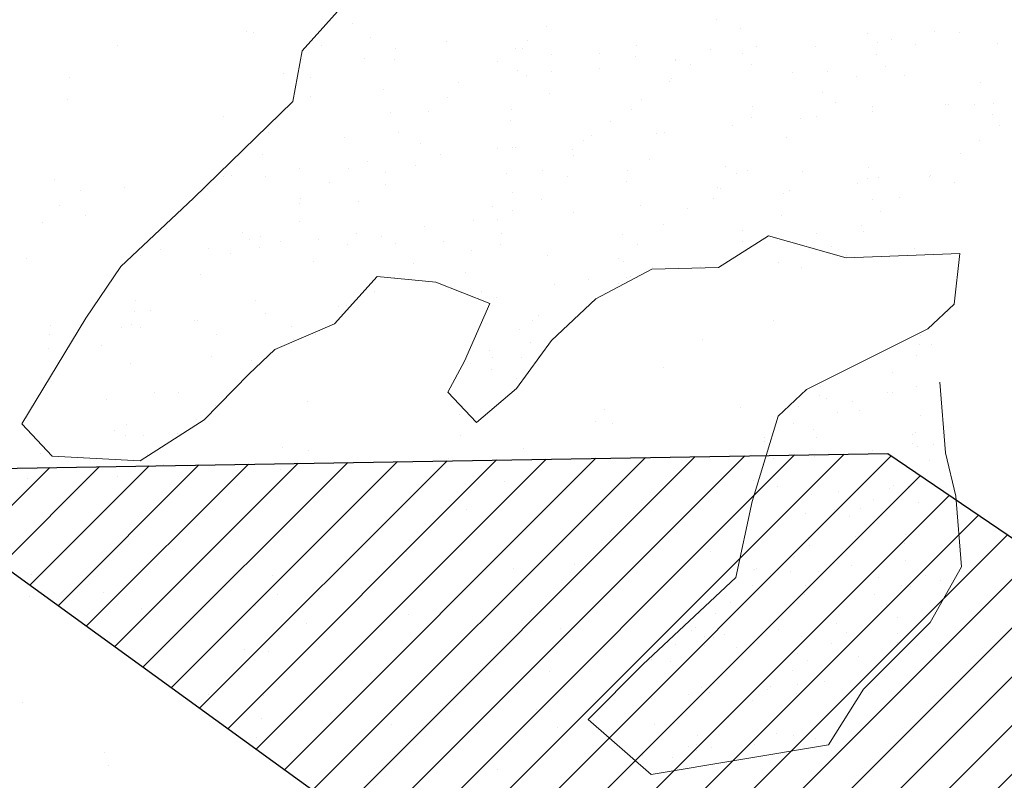
# Model space of a CAD drawing. Units: inches. Extents: x 1986 to 21484, y -1816 to 2016.
# Tile 61 of 85: x 3651.423 to 3655.81, y 1889.501 to 1892.891. Entities that reach past the tile are written whole.
import ezdxf

# ---------------------------------------------------------------- set-up
doc = ezdxf.new("R2010")
doc.units = ezdxf.units.IN
doc.layers.add('L-PLNT', color=84, linetype='Continuous', lineweight=13)
doc.layers.add('vfolha2', color=110, linetype='Continuous')

# ---------------------------------------------------------------- blocks, each defined once
blk = doc.blocks.new('arbusto_PB_verde_grande')
at = {"layer": 'vfolha2'}
h = blk.add_hatch(dxfattribs=at)
h.set_pattern_fill('ANSI31', color=256, scale=0.05, style=0)
h.set_pattern_definition([(45, (-2446.5133113, 50.986076), (-0.004419417382, 0.004419417382), [])])
h.paths.add_polyline_path([(0.02944, 0.35651), (0.00028, 0.09048), (0.02625, -0.03934), (0.047, 0.06233), (0.06189, 0.09731), (0.09372, 0.26573), (0.09955, 0.43473), (0.08789, 0.61313), (0.0645, 0.72266), (0.04988, 0.6851), (0.0236, 0.51294)])
h.paths.add_polyline_path([(0.30106, 0.43789), (0.14225, 0.24871), (0.26685, 0.30022)])
h.paths.add_polyline_path([(0.37995, 0.22817), (0.23697, 0.15193), (0.18428, 0.09364), (0.11122, 0.04358), (0.02625, -0.03934), (0.28061, 0.04667), (0.36829, 0.07798), (0.46756, 0.11239), (0.61068, 0.19376), (0.71585, 0.27823), (0.55813, 0.25948)])
h.paths.add_polyline_path([(0.56101, -0.29441), (0.72752, -0.32573), (0.59024, -0.2412), (0.42962, -0.15982), (0.02625, -0.03934), (0.14922, -0.14107), (0.18838, -0.16604), (0.41501, -0.24435)])
h.paths.add_polyline_path([(-0.27429, -0.44776), (-0.30352, -0.72628), (-0.23923, -0.64175), (-0.15457, -0.45716), (0.02625, -0.03934), (-0.16328, -0.25376)])
h.paths.add_polyline_path([(-0.51963, -0.24744), (-0.67736, -0.32573), (-0.59558, -0.35072), (-0.40574, -0.32882), (-0.21007, -0.20995), (0.02625, -0.03934), (-0.14874, -0.06595), (-0.31518, -0.09101), (-0.41452, -0.15048)])
h.paths.add_polyline_path([(-0.52546, 0.25007), (-0.70947, 0.24698), (-0.51963, 0.1093), (-0.32979, 0.02167), (-0.07567, -0.0128), (-0.04234, -0.02148), (-0.35024, 0.1312)])
for p, q in [((-0.70947, 0.24698), (-0.52546, 0.25007)), ((-0.52546, 0.25007), (-0.35024, 0.1312)), ((-0.51963, 0.1093), (-0.70947, 0.24698))]:
    blk.add_line(p, q, dxfattribs=at)
blk = doc.blocks.new('PLANT-SHRUB')
for p, q in [((2170.2504, 1876.25), (2169.9665, 1876.176)), ((2170.9168, 1875.8061), (2170.2504, 1876.25)), ((2169.9665, 1876.176), (2169.5469, 1876.1637)), ((2170.2731, 1876.1911), (2170.2731, 1876.1911)), ((2169.5469, 1876.1637), (2169.2754, 1876.0773)), ((2169.5469, 1876.1637), (2169.5469, 1876.1637)), ((2169.7163, 1876.1281), (2169.7163, 1876.1281)), ((2169.6868, 1876.1011), (2169.6868, 1876.1011)), ((2170.336, 1876.1153), (2170.336, 1876.1153)), ((2169.2754, 1876.0773), (2169.0779, 1875.8307)), ((2169.387, 1876.0573), (2169.387, 1876.0573)), ((2169.6384, 1876.0466), (2169.6384, 1876.0466)), ((2169.8848, 1876.0564), (2169.8848, 1876.0564)), ((2170.3827, 1876.0555), (2170.3827, 1876.0555)), ((2169.4198, 1875.9977), (2169.4198, 1875.9977)), ((2170.0702, 1876.031), (2170.0702, 1876.031)), ((2170.4887, 1876.0257), (2170.4887, 1876.0257)), ((2169.503, 1875.9867), (2169.503, 1875.9867)), ((2169.5277, 1875.9553), (2169.5277, 1875.9553)), ((2169.633, 1875.9696), (2169.633, 1875.9696)), ((2170.1674, 1875.9608), (2170.1674, 1875.9608)), ((2170.1969, 1875.9878), (2170.1969, 1875.9878)), ((2169.8501, 1875.941), (2169.8501, 1875.941)), ((2169.9334, 1875.9301), (2169.9334, 1875.9301)), ((2170.0633, 1875.913), (2170.0633, 1875.913)), ((2169.4356, 1875.8865), (2169.4356, 1875.8865)), ((2169.6421, 1875.9018), (2169.6421, 1875.9018)), ((2169.8541, 1875.8811), (2169.8541, 1875.8811)), ((2170.14, 1875.9009), (2170.14, 1875.9009)), ((2170.263, 1875.8831), (2170.263, 1875.8831)), ((2170.2805, 1875.8844), (2170.2805, 1875.8844)), ((2170.3637, 1875.8734), (2170.3637, 1875.8734)), ((2170.6378, 1875.9), (2170.6378, 1875.9)), ((2170.6948, 1875.8675), (2170.6948, 1875.8675)), ((2169.0779, 1875.8307), (2168.9792, 1875.6581)), ((2169.3886, 1875.8279), (2169.3886, 1875.8279)), ((2169.5747, 1875.8588), (2169.5747, 1875.8588)), ((2170.0725, 1875.8579), (2170.0725, 1875.8579)), ((2170.4937, 1875.8563), (2170.4937, 1875.8563)), ((2170.5704, 1875.857), (2170.5704, 1875.857)), ((2170.648, 1875.8205), (2170.648, 1875.8205)), ((2170.6775, 1875.8475), (2170.6775, 1875.8475)), ((2170.7108, 1875.8277), (2170.7108, 1875.8277)), ((2169.3592, 1875.8009), (2169.3592, 1875.8009)), ((2170.0083, 1875.815), (2170.0083, 1875.815)), ((2170.794, 1875.8168), (2170.794, 1875.8168)), ((2170.9538, 1875.4361), (2170.9168, 1875.8061)), ((2169.2194, 1875.7366), (2169.2194, 1875.7366)), ((2169.6284, 1875.7385), (2169.6284, 1875.7385)), ((2169.8692, 1875.6876), (2169.8692, 1875.6876)), ((2170.0602, 1875.723), (2170.0602, 1875.723)), ((2170.4786, 1875.7176), (2170.4786, 1875.7176)), ((2170.8876, 1875.7196), (2170.8876, 1875.7196)), ((2168.9792, 1875.6581), (2168.7818, 1875.4114)), ((2169.2001, 1875.6551), (2169.2001, 1875.6551)), ((2169.2578, 1875.657), (2169.2578, 1875.657)), ((2169.5298, 1875.6563), (2169.5298, 1875.6563)), ((2169.7557, 1875.6561), (2169.7557, 1875.6561)), ((2169.8398, 1875.6606), (2169.8398, 1875.6606)), ((2170.2535, 1875.6552), (2170.2535, 1875.6552)), ((2170.4889, 1875.6747), (2170.4889, 1875.6747)), ((2170.5522, 1875.6612), (2170.5522, 1875.6612)), ((2170.7514, 1875.6543), (2170.7514, 1875.6543)), ((2169.0553, 1875.6318), (2169.0553, 1875.6318)), ((2169.2502, 1875.6061), (2169.2502, 1875.6061)), ((2169.2724, 1875.6032), (2169.2724, 1875.6032)), ((2168.9937, 1875.594), (2168.9937, 1875.594)), ((2169.3556, 1875.5922), (2169.3556, 1875.5922)), ((2169.4255, 1875.5784), (2169.4255, 1875.5784)), ((2169.4856, 1875.5751), (2169.4856, 1875.5751)), ((2169.844, 1875.5731), (2169.844, 1875.5731)), ((2170.2529, 1875.575), (2170.2529, 1875.575)), ((2170.6847, 1875.5595), (2170.6847, 1875.5595)), ((2169.05, 1875.5534), (2169.05, 1875.5534)), ((2169.061, 1875.5276), (2169.061, 1875.5276)), ((2169.6806, 1875.5148), (2169.6806, 1875.5148)), ((2169.7027, 1875.5465), (2169.7027, 1875.5465)), ((2169.786, 1875.5356), (2169.786, 1875.5356)), ((2169.7931, 1875.5346), (2169.7931, 1875.5346)), ((2169.9159, 1875.5185), (2169.9159, 1875.5185)), ((2170.2946, 1875.5512), (2170.2946, 1875.5512)), ((2170.3203, 1875.5203), (2170.3203, 1875.5203)), ((2170.3498, 1875.5473), (2170.3498, 1875.5473)), ((2169.0151, 1875.5024), (2169.0151, 1875.5024)), ((2169.0315, 1875.5006), (2169.0315, 1875.5006)), ((2169.513, 1875.5015), (2169.513, 1875.5015)), ((2170.0108, 1875.5005), (2170.0108, 1875.5005)), ((2170.1331, 1875.4899), (2170.1331, 1875.4899)), ((2170.2163, 1875.4789), (2170.2163, 1875.4789)), ((2170.5087, 1875.4996), (2170.5087, 1875.4996)), ((2168.9477, 1875.4594), (2168.9477, 1875.4594)), ((2169.2093, 1875.4285), (2169.2093, 1875.4285)), ((2169.4456, 1875.4585), (2169.4456, 1875.4585)), ((2169.6183, 1875.4305), (2169.6183, 1875.4305)), ((2169.7567, 1875.2265), (2170.0406, 1875.4238)), ((2169.9434, 1875.4576), (2169.9434, 1875.4576)), ((2169.9553, 1875.456), (2169.9553, 1875.456)), ((2170.0406, 1875.4238), (2170.6083, 1875.4238)), ((2170.326, 1875.4645), (2170.326, 1875.4645)), ((2170.3463, 1875.4618), (2170.3463, 1875.4618)), ((2170.4413, 1875.4567), (2170.4413, 1875.4567)), ((2170.5634, 1875.4332), (2170.5634, 1875.4332)), ((2170.6083, 1875.4238), (2170.9538, 1875.4361)), ((2170.9391, 1875.4558), (2170.9391, 1875.4558)), ((2169.5416, 1875.3873), (2169.5416, 1875.3873)), ((2170.8689, 1875.393), (2170.8689, 1875.393)), ((2168.8724, 1875.3548), (2168.8724, 1875.3548)), ((2169.5121, 1875.3603), (2169.5121, 1875.3603)), ((2171.0769, 1875.3656), (2171.0769, 1875.3656)), ((2168.9656, 1875.2998), (2168.9656, 1875.2998)), ((2171.4019, 1875.3228), (2171.4019, 1875.3228)), ((2168.6947, 1875.2653), (2168.6947, 1875.2653)), ((2168.7779, 1875.2544), (2168.7779, 1875.2544)), ((2168.9837, 1875.2859), (2168.9837, 1875.2859)), ((2169.1287, 1875.2566), (2169.1287, 1875.2566)), ((2169.4154, 1875.2704), (2169.4154, 1875.2704)), ((2169.6266, 1875.2557), (2169.6266, 1875.2557)), ((2170.0451, 1875.2609), (2170.0451, 1875.2609)), ((2171.0912, 1875.2476), (2171.0912, 1875.2476)), ((2168.7333, 1875.2274), (2168.7333, 1875.2274)), ((2168.9079, 1875.2372), (2168.9079, 1875.2372)), ((2169.125, 1875.2087), (2169.125, 1875.2087)), ((2169.353, 1875.2145), (2169.353, 1875.2145)), ((2169.4112, 1875.0292), (2169.7567, 1875.2265)), ((2168.3251, 1875.0538), (2168.4979, 1875.2018)), ((2168.4979, 1875.2018), (2168.6583, 1875.2018)), ((2168.6583, 1875.2018), (2169.2384, 1875.0292)), ((2168.7038, 1875.2004), (2168.7038, 1875.2004)), ((2169.2082, 1875.1977), (2169.2082, 1875.1977)), ((2169.3382, 1875.1806), (2169.3382, 1875.1806)), ((2169.6879, 1875.1646), (2169.6879, 1875.1646)), ((2170.9325, 1875.1624), (2170.9325, 1875.1624)), ((2169.1993, 1875.1205), (2169.1993, 1875.1205)), ((2169.5553, 1875.152), (2169.5553, 1875.152)), ((2169.6075, 1875.1374), (2169.6075, 1875.1374)), ((2169.2139, 1875.0871), (2169.2139, 1875.0871)), ((2169.3839, 1875.1011), (2169.3839, 1875.1011)), ((2171.1567, 1875.1052), (2171.1567, 1875.1052)), ((2168.3251, 1875.0538), (2168.3251, 1875.0538)), ((2168.7077, 1874.7209), (2168.3251, 1875.0538)), ((2169.1844, 1875.0601), (2169.1844, 1875.0601)), ((2169.2384, 1875.0292), (2169.4112, 1875.0292)), ((2169.3165, 1875.0582), (2169.3165, 1875.0582)), ((2169.5194, 1875.0573), (2169.5194, 1875.0573)), ((2169.5339, 1875.0699), (2169.5339, 1875.0699)), ((2170.764, 1875.055), (2170.764, 1875.055)), ((2168.4584, 1874.8995), (2168.4584, 1874.8995)), ((2168.4584, 1874.8995), (2168.4584, 1874.8995)), ((2169.5046, 1874.8862), (2169.5046, 1874.8862)), ((2170.527, 1874.8911), (2170.527, 1874.8911)), ((2171.6065, 1874.8522), (2171.6065, 1874.8522)), ((2168.1245, 1874.8072), (2168.1245, 1874.8072)), ((2170.809, 1874.7866), (2170.809, 1874.7866)), ((2167.8059, 1874.7614), (2167.8059, 1874.7614)), ((2167.9149, 1874.7471), (2167.9149, 1874.7471)), ((2168.0189, 1874.7334), (2168.0189, 1874.7334)), ((2168.8928, 1874.4126), (2168.7077, 1874.7209)), ((2167.7959, 1874.7038), (2167.7959, 1874.7038)), ((2168.1814, 1874.712), (2168.1814, 1874.712)), ((2168.1882, 1874.7122), (2168.1882, 1874.7122)), ((2168.3488, 1874.69), (2168.3488, 1874.69)), ((2168.5705, 1874.6877), (2168.5705, 1874.6877)), ((2168.6994, 1874.7146), (2168.6994, 1874.7146)), ((2169.1361, 1874.7054), (2169.1361, 1874.7054)), ((2170.7353, 1874.7191), (2170.7353, 1874.7191)), ((2167.759, 1874.67), (2167.759, 1874.67)), ((2168.4528, 1874.6763), (2168.4528, 1874.6763)), ((2168.5568, 1874.6626), (2168.5568, 1874.6626)), ((2168.5568, 1874.6626), (2168.5568, 1874.6626)), ((2168.7193, 1874.6412), (2168.7193, 1874.6412)), ((2167.8211, 1874.6139), (2167.8211, 1874.6139)), ((2168.4434, 1874.6128), (2168.4434, 1874.6128)), ((2168.8817, 1874.6198), (2168.8817, 1874.6198)), ((2167.7368, 1874.5603), (2167.7368, 1874.5603)), ((2168.3591, 1874.5591), (2168.3591, 1874.5591)), ((2168.7272, 1874.5526), (2168.7272, 1874.5526)), ((2169.4246, 1874.5483), (2169.4246, 1874.5483)), ((2169.9719, 1874.5504), (2169.9719, 1874.5504)), ((2171.2165, 1874.5481), (2171.2165, 1874.5481)), ((2167.9061, 1874.5339), (2167.9061, 1874.5339)), ((2167.918, 1874.5248), (2167.918, 1874.5248)), ((2168.3966, 1874.5284), (2168.3966, 1874.5284)), ((2168.4459, 1874.5145), (2168.4459, 1874.5145)), ((2168.9404, 1874.5297), (2168.9404, 1874.5297)), ((2169.6326, 1874.5209), (2169.6326, 1874.5209)), ((2167.5601, 1874.4878), (2167.5601, 1874.4878)), ((2168.3598, 1874.4946), (2168.3598, 1874.4946)), ((2169.9576, 1874.4782), (2169.9576, 1874.4782)), ((2170.0199, 1874.4908), (2170.0199, 1874.4908)), ((2171.0661, 1874.4775), (2171.0661, 1874.4775)), ((2172.0884, 1874.4824), (2172.0884, 1874.4824)), ((2172.0105, 1874.4358), (2172.0105, 1874.4358)), ((2168.7884, 1874.3867), (2168.7884, 1874.3867)), ((2169.152, 1874.3632), (2168.8928, 1874.4126)), ((2170.5004, 1874.4067), (2170.5004, 1874.4067)), ((2170.7085, 1874.3793), (2170.7085, 1874.3793)), ((2167.6526, 1874.3338), (2167.6526, 1874.3338)), ((2168.1756, 1874.3271), (2168.1756, 1874.3271)), ((2168.6868, 1874.3296), (2168.6868, 1874.3296)), ((2168.9973, 1874.353), (2168.9973, 1874.353)), ((2169.3741, 1874.1659), (2169.152, 1874.3632)), ((2170.3375, 1874.3546), (2170.3375, 1874.3546)), ((2171.0334, 1874.3365), (2171.0334, 1874.3365)), ((2171.9368, 1874.3683), (2171.9368, 1874.3683)), ((2167.9631, 1874.3068), (2167.9631, 1874.3068)), ((2168.1609, 1874.3124), (2168.1609, 1874.3124)), ((2168.5854, 1874.3057), (2168.5854, 1874.3057)), ((2168.7147, 1874.3192), (2168.7147, 1874.3192)), ((2168.9605, 1874.3192), (2168.9605, 1874.3192)), ((2169.2077, 1874.3045), (2169.2077, 1874.3045)), ((2167.7306, 1874.2539), (2167.7306, 1874.2539)), ((2167.8346, 1874.2402), (2167.8346, 1874.2402)), ((2171.5762, 1874.2651), (2171.5762, 1874.2651)), ((2167.9971, 1874.2189), (2167.9971, 1874.2189)), ((2171.7843, 1874.2377), (2171.7843, 1874.2377)), ((2172.1092, 1874.1949), (2172.1092, 1874.1949)), ((2167.987, 1874.1531), (2167.987, 1874.1531)), ((2168.1205, 1874.1661), (2168.1205, 1874.1661)), ((2168.2685, 1874.1831), (2168.2685, 1874.1831)), ((2168.3726, 1874.1694), (2168.3726, 1874.1694)), ((2169.3651, 1874.1638), (2169.3651, 1874.1638)), ((2169.6456, 1874.0919), (2169.3741, 1874.1659)), ((2170.6097, 1874.1616), (2170.6097, 1874.1616)), ((2171.8544, 1874.1593), (2171.8544, 1874.1593)), ((2167.8935, 1874.1489), (2167.8935, 1874.1489)), ((2167.9502, 1874.1193), (2167.9502, 1874.1193)), ((2168.282, 1874.1124), (2168.282, 1874.1124)), ((2168.4333, 1874.1294), (2168.4333, 1874.1294)), ((2168.4333, 1874.1294), (2168.4333, 1874.1294)), ((2168.535, 1874.148), (2168.535, 1874.148)), ((2168.7616, 1874.137), (2168.7616, 1874.137)), ((2168.8065, 1874.1123), (2168.8065, 1874.1123)), ((2168.9043, 1874.1113), (2168.9043, 1874.1113)), ((2168.9564, 1874.1228), (2168.9564, 1874.1228)), ((2169.4676, 1874.1252), (2169.4676, 1874.1252)), ((2169.4794, 1874.1161), (2169.4794, 1874.1161)), ((2169.5266, 1874.1101), (2169.5266, 1874.1101)), ((2170.1763, 1874.1413), (2169.9172, 1874.0919)), ((2170.149, 1874.109), (2170.149, 1874.109)), ((2170.4108, 1874.1289), (2170.1763, 1874.1413)), ((2170.4108, 1874.1289), (2170.4108, 1874.1289)), ((2170.4108, 1873.944), (2170.4108, 1874.1289)), ((2170.5018, 1874.121), (2170.5018, 1874.121)), ((2172.6521, 1874.1234), (2172.6521, 1874.1234)), ((2168.9105, 1874.0986), (2168.9105, 1874.0986)), ((2169.0729, 1874.0772), (2169.0729, 1874.0772)), ((2169.9172, 1874.0919), (2169.6456, 1874.0919)), ((2170.0073, 1874.1058), (2170.0073, 1874.1058)), ((2171.5813, 1874.0821), (2171.5813, 1874.0821)), ((2172.6275, 1874.0688), (2172.6275, 1874.0688)), ((2167.9519, 1874.0587), (2167.9519, 1874.0587)), ((2168.1977, 1874.0587), (2168.1977, 1874.0587)), ((2168.8201, 1874.0576), (2168.8201, 1874.0576)), ((2169.1966, 1874.0565), (2169.1966, 1874.0565)), ((2169.3444, 1874.0415), (2169.3444, 1874.0415)), ((2169.4424, 1874.0565), (2169.4424, 1874.0565)), ((2169.4484, 1874.0278), (2169.4484, 1874.0278)), ((2169.9898, 1874.036), (2169.9898, 1874.036)), ((2170.0647, 1874.0553), (2170.0647, 1874.0553)), ((2170.4412, 1874.0542), (2170.4412, 1874.0542)), ((2171.6858, 1874.0519), (2171.6858, 1874.0519)), ((2168.5877, 1873.9777), (2168.5877, 1873.9777)), ((2169.6108, 1874.0064), (2169.6108, 1874.0064)), ((2170.1988, 1874.0022), (2170.1988, 1874.0022)), ((2171.539, 1874.0038), (2171.539, 1874.0038)), ((2168.1631, 1873.9421), (2168.1631, 1873.9421)), ((2168.3169, 1873.9547), (2168.3169, 1873.9547)), ((2168.5509, 1873.9439), (2168.5509, 1873.9439)), ((2168.6742, 1873.9445), (2168.6742, 1873.9445)), ((2169.3623, 1873.9616), (2169.3623, 1873.9616)), ((2169.8823, 1873.9707), (2169.8823, 1873.9707)), ((2169.9162, 1873.9685), (2169.9162, 1873.9685)), ((2169.9863, 1873.957), (2169.9863, 1873.957)), ((2170.1488, 1873.9356), (2170.1488, 1873.9356)), ((2170.162, 1873.9685), (2170.162, 1873.9685)), ((2170.2627, 1873.8946), (2170.4108, 1873.944)), ((2169.214, 1873.9251), (2169.214, 1873.9251)), ((2169.7371, 1873.9184), (2169.7371, 1873.9184)), ((2170.0035, 1873.7837), (2170.2627, 1873.8946)), ((2170.2483, 1873.9209), (2170.2483, 1873.9209)), ((2168.424, 1873.8053), (2168.424, 1873.8053)), ((2169.0463, 1873.8041), (2169.0463, 1873.8041)), ((2169.1885, 1873.8023), (2169.1885, 1873.8023)), ((2169.6686, 1873.803), (2169.6686, 1873.803)), ((2168.352, 1873.7617), (2168.352, 1873.7617)), ((2168.9152, 1873.7596), (2168.9152, 1873.7596)), ((2169.1516, 1873.7685), (2169.1516, 1873.7685)), ((2169.9631, 1873.7862), (2169.9631, 1873.7862)), ((2170.1146, 1873.5494), (2170.0035, 1873.7837)), ((2168.4207, 1873.7444), (2168.4207, 1873.7444)), ((2168.9438, 1873.7377), (2168.9438, 1873.7377)), ((2169.455, 1873.7402), (2169.455, 1873.7402)), ((2169.9947, 1873.7207), (2169.9947, 1873.7207)), ((2169.9947, 1873.7207), (2169.9947, 1873.7207)), ((2172.0633, 1873.7123), (2172.0633, 1873.7123)), ((2171.0409, 1873.7074), (2171.0409, 1873.7074)), ((2171.1913, 1873.6852), (2171.1913, 1873.6852)), ((2168.3508, 1873.6549), (2168.3508, 1873.6549)), ((2168.5132, 1873.6335), (2168.5132, 1873.6335)), ((2169.7892, 1873.6269), (2169.7892, 1873.6269)), ((2172.7405, 1873.653), (2172.7405, 1873.653)), ((2168.6222, 1873.6192), (2168.6222, 1873.6192)), ((2168.7262, 1873.6055), (2168.7262, 1873.6055)), ((2168.7429, 1873.6109), (2168.7429, 1873.6109)), ((2168.8887, 1873.5841), (2168.8887, 1873.5841)), ((2168.9527, 1873.5863), (2168.9527, 1873.5863)), ((2169.3653, 1873.6097), (2169.3653, 1873.6097)), ((2169.5184, 1873.6039), (2169.5184, 1873.6039)), ((2169.7524, 1873.5931), (2169.7524, 1873.5931)), ((2169.9876, 1873.6086), (2169.9876, 1873.6086)), ((2171.1176, 1873.6177), (2171.1176, 1873.6177)), ((2168.4044, 1873.5518), (2168.4044, 1873.5518)), ((2168.6587, 1873.5572), (2168.6587, 1873.5572)), ((2168.6617, 1873.5595), (2168.6617, 1873.5595)), ((2169.0561, 1873.562), (2169.0561, 1873.562)), ((2169.1601, 1873.5483), (2169.1601, 1873.5483)), ((2169.2014, 1873.54), (2169.2014, 1873.54)), ((2169.281, 1873.556), (2169.281, 1873.556)), ((2169.6491, 1873.5495), (2169.6491, 1873.5495)), ((2169.9033, 1873.5549), (2169.9033, 1873.5549)), ((2170.1146, 1873.5494), (2170.1146, 1873.5494)), ((2170.2874, 1873.352), (2170.1146, 1873.5494)), ((2170.8937, 1873.5473), (2170.8937, 1873.5473)), ((2172.1383, 1873.545), (2172.1383, 1873.545)), ((2169.2641, 1873.5346), (2169.2641, 1873.5346)), ((2169.2641, 1873.5346), (2169.2641, 1873.5346)), ((2169.4266, 1873.5133), (2169.4266, 1873.5133)), ((2169.7245, 1873.5334), (2169.7245, 1873.5334)), ((2169.5891, 1873.4919), (2169.5891, 1873.4919)), ((2169.698, 1873.4775), (2169.698, 1873.4775)), ((2169.802, 1873.4638), (2169.802, 1873.4638)), ((2168.7789, 1873.427), (2168.7789, 1873.427)), ((2169.5535, 1873.4109), (2169.5535, 1873.4109)), ((2169.9645, 1873.4424), (2169.9645, 1873.4424)), ((2170.1319, 1873.4204), (2170.1319, 1873.4204)), ((2170.2359, 1873.4067), (2170.2359, 1873.4067)), ((2168.742, 1873.3932), (2168.742, 1873.3932)), ((2170.5712, 1873.3767), (2170.2874, 1873.352)), ((2170.34, 1873.393), (2170.34, 1873.393)), ((2170.8427, 1873.2781), (2170.5712, 1873.3767)), ((2168.9312, 1873.3527), (2168.9312, 1873.3527)), ((2169.4424, 1873.3551), (2169.4424, 1873.3551)), ((2169.4543, 1873.346), (2169.4543, 1873.346)), ((2169.9821, 1873.3357), (2169.9821, 1873.3357)), ((2170.4767, 1873.3509), (2170.4767, 1873.3509)), ((2170.5052, 1873.329), (2170.5052, 1873.329)), ((2170.6649, 1873.3502), (2170.6649, 1873.3502)), ((2172.3928, 1873.3344), (2172.3928, 1873.3344)), ((2168.8849, 1873.3037), (2168.8849, 1873.3037)), ((2169.1706, 1873.2853), (2169.1706, 1873.2853)), ((2169.5072, 1873.3026), (2169.5072, 1873.3026)), ((2170.1295, 1873.3015), (2170.1295, 1873.3015)), ((2170.7519, 1873.3003), (2170.7519, 1873.3003)), ((2171.0032, 1873.2781), (2170.8427, 1873.2781)), ((2170.9907, 1873.2761), (2170.9907, 1873.2761)), ((2171.287, 1873.2904), (2171.0032, 1873.2781)), ((2171.2077, 1873.2788), (2171.2077, 1873.2788)), ((2171.6202, 1873.2287), (2171.287, 1873.2904)), ((2171.5561, 1873.312), (2171.5561, 1873.312)), ((2169.3796, 1873.2516), (2169.3796, 1873.2516)), ((2170.1542, 1873.2355), (2170.1542, 1873.2355)), ((2170.7198, 1873.2532), (2170.7198, 1873.2532)), ((2170.9538, 1873.2424), (2170.9538, 1873.2424)), ((2171.3118, 1873.2651), (2171.3118, 1873.2651)), ((2171.4158, 1873.2514), (2171.4158, 1873.2514)), ((2171.4158, 1873.2514), (2171.4158, 1873.2514)), ((2171.5782, 1873.23), (2171.5782, 1873.23)), ((2172.3191, 1873.2669), (2172.3191, 1873.2669)), ((2169.097, 1873.2178), (2169.097, 1873.2178)), ((2169.3428, 1873.2178), (2169.3428, 1873.2178)), ((2171.8918, 1872.9451), (2171.6202, 1873.2287)), ((2171.7407, 1873.2086), (2171.7407, 1873.2086)), ((2169.0423, 1873.163), (2169.0423, 1873.163)), ((2169.1888, 1873.155), (2169.1888, 1873.155)), ((2169.7119, 1873.1483), (2169.7119, 1873.1483)), ((2170.2231, 1873.1508), (2170.2231, 1873.1508)), ((2170.287, 1873.1607), (2170.287, 1873.1607)), ((2171.5316, 1873.1585), (2171.5316, 1873.1585)), ((2169.2039, 1873.1093), (2169.2039, 1873.1093)), ((2169.8262, 1873.1082), (2169.8262, 1873.1082)), ((2170.4485, 1873.1071), (2170.4485, 1873.1071)), ((2170.7628, 1873.1313), (2170.7628, 1873.1313)), ((2171.0708, 1873.1059), (2171.0708, 1873.1059)), ((2171.2859, 1873.1247), (2171.2859, 1873.1247)), ((2171.5914, 1873.1007), (2171.5914, 1873.1007)), ((2168.9759, 1873.0552), (2168.9759, 1873.0552)), ((2169.1196, 1873.0556), (2169.1196, 1873.0556)), ((2169.7419, 1873.0545), (2169.7419, 1873.0545)), ((2169.9803, 1873.0762), (2169.9803, 1873.0762)), ((2170.1184, 1873.0534), (2170.1184, 1873.0534)), ((2170.3642, 1873.0534), (2170.3642, 1873.0534)), ((2170.7549, 1873.0601), (2170.7549, 1873.0601)), ((2171.5546, 1873.067), (2171.5546, 1873.067)), ((2169.0799, 1873.0415), (2169.0799, 1873.0415)), ((2169.1439, 1873.0356), (2169.1439, 1873.0356)), ((2169.2423, 1873.0201), (2169.2423, 1873.0201)), ((2169.9435, 1873.0424), (2169.9435, 1873.0424)), ((2170.9865, 1873.0522), (2170.9865, 1873.0522)), ((2171.3631, 1873.0511), (2171.3631, 1873.0511)), ((2171.6089, 1873.0511), (2171.6089, 1873.0511)), ((2169.4298, 1872.9701), (2169.4298, 1872.9701)), ((2169.5138, 1872.9844), (2169.5138, 1872.9844)), ((2169.6178, 1872.9707), (2169.6178, 1872.9707)), ((2169.7803, 1872.9493), (2169.7803, 1872.9493)), ((2169.9695, 1872.9506), (2169.9695, 1872.9506)), ((2169.9695, 1872.9506), (2169.9695, 1872.9506)), ((2170.3721, 1872.9345), (2170.3721, 1872.9345)), ((2170.4926, 1872.944), (2170.4926, 1872.944)), ((2171.0038, 1872.9464), (2171.0038, 1872.9464)), ((2171.0157, 1872.9373), (2171.0157, 1872.9373)), ((2171.5435, 1872.927), (2171.5435, 1872.927)), ((2171.8918, 1872.7478), (2171.8918, 1872.9451)), ((2172.0381, 1872.9422), (2172.0381, 1872.9422)), ((2170.0517, 1872.9136), (2170.0517, 1872.9136)), ((2170.1557, 1872.8999), (2170.1557, 1872.8999)), ((2170.3182, 1872.8785), (2170.3182, 1872.8785)), ((2170.5811, 1872.9008), (2170.5811, 1872.9008)), ((2171.3557, 1872.8847), (2171.3557, 1872.8847)), ((2171.9213, 1872.9024), (2171.9213, 1872.9024)), ((2169.7446, 1872.8602), (2169.7446, 1872.8602)), ((2170.2984, 1872.867), (2170.2984, 1872.867)), ((2170.5442, 1872.867), (2170.5442, 1872.867)), ((2170.5896, 1872.8427), (2170.5896, 1872.8427)), ((2169.3458, 1872.8022), (2169.3458, 1872.8022)), ((2169.9682, 1872.8011), (2169.9682, 1872.8011)), ((2170.5905, 1872.7999), (2170.5905, 1872.7999)), ((2170.6936, 1872.829), (2170.6936, 1872.829)), ((2170.8561, 1872.8077), (2170.8561, 1872.8077)), ((2171.2128, 1872.7988), (2171.2128, 1872.7988)), ((2169.6993, 1872.7633), (2169.6993, 1872.7633)), ((2170.2105, 1872.7657), (2170.2105, 1872.7657)), ((2170.7502, 1872.7463), (2170.7502, 1872.7463)), ((2171.1275, 1872.7719), (2171.1275, 1872.7719)), ((2171.2315, 1872.7582), (2171.2315, 1872.7582)), ((2171.3611, 1872.5998), (2171.8918, 1872.7478)), ((2171.1818, 1872.7254), (2171.1818, 1872.7254)), ((2171.2733, 1872.7396), (2171.2733, 1872.7396)), ((2171.394, 1872.7368), (2171.394, 1872.7368)), ((2169.5339, 1872.6671), (2169.5339, 1872.6671)), ((2169.5708, 1872.7009), (2169.5708, 1872.7009)), ((2170.3453, 1872.6848), (2170.3453, 1872.6848)), ((2171.145, 1872.6916), (2171.145, 1872.6916)), ((2171.6654, 1872.7011), (2171.6654, 1872.7011)), ((2169.6648, 1872.6078), (2169.6648, 1872.6078)), ((2170.2871, 1872.6067), (2170.2871, 1872.6067)), ((2170.4515, 1872.5808), (2170.4515, 1872.5808)), ((2170.9094, 1872.6055), (2170.9094, 1872.6055)), ((2171.0896, 1872.5382), (2171.3611, 1872.5998)), ((2171.5736, 1872.5838), (2171.5736, 1872.5838)), ((2169.5805, 1872.5541), (2169.5805, 1872.5541)), ((2169.9569, 1872.5656), (2169.9569, 1872.5656)), ((2170.0282, 1872.5258), (2170.6453, 1872.5382)), ((2170.2028, 1872.553), (2170.2028, 1872.553)), ((2170.48, 1872.5589), (2170.48, 1872.5589)), ((2170.5709, 1872.5465), (2170.5709, 1872.5465)), ((2170.6453, 1872.5382), (2171.0896, 1872.5382)), ((2170.8251, 1872.5518), (2170.8251, 1872.5518)), ((2170.9912, 1872.5614), (2170.9912, 1872.5614)), ((2171.531, 1872.5419), (2171.531, 1872.5419)), ((2169.8431, 1872.3902), (2170.0282, 1872.5258)), ((2169.9006, 1872.5025), (2169.9006, 1872.5025)), ((2171.4999, 1872.5163), (2171.4999, 1872.5163)), ((2169.596, 1872.4561), (2169.596, 1872.4561)), ((2169.7634, 1872.4341), (2169.7634, 1872.4341)), ((2169.8674, 1872.4204), (2169.8674, 1872.4204)), ((2169.9715, 1872.4067), (2169.9715, 1872.4067)), ((2169.2754, 1872.3408), (2169.8431, 1872.3902)), ((2169.6867, 1872.3782), (2169.6867, 1872.3782)), ((2170.2964, 1872.3639), (2170.2964, 1872.3639)), ((2170.8393, 1872.2925), (2170.8393, 1872.2925)), ((2171.0473, 1872.2651), (2171.0473, 1872.2651)), ((2171.3722, 1872.2223), (2171.3722, 1872.2223)), ((2169.9443, 1872.1805), (2169.9443, 1872.1805)), ((2169.9642, 1872.1599), (2169.9642, 1872.1599)), ((2170.9905, 1872.1672), (2170.9905, 1872.1672)), ((2171.1021, 1872.1517), (2171.1021, 1872.1517)), ((2171.2088, 1872.1577), (2171.2088, 1872.1577)), ((2171.0403, 1872.0503), (2171.0403, 1872.0503)), ((2170.7544, 1871.8331), (2170.7544, 1871.8331)), ((2170.4263, 1871.8107), (2170.4263, 1871.8107)), ((2170.6807, 1871.7656), (2170.6807, 1871.7656))]:
    blk.add_line(p, q)

msp = doc.modelspace()

# ---------------------------------------------------------------- block references
at = {"layer": 'L-PLNT', "rotation": 223.1883365522388}
msp.add_blockref('PLANT-SHRUB', (3953.27, 4742.9646), dxfattribs=at)
at = {"layer": 'L-PLNT', "xscale": 24.60366729364114, "yscale": 24.60366729364114, "zscale": 24.60366729364114}
msp.add_blockref('arbusto_PB_verde_grande', (3668.2184, 1884.8051), dxfattribs=at)

doc.saveas('drawing.dxf')
